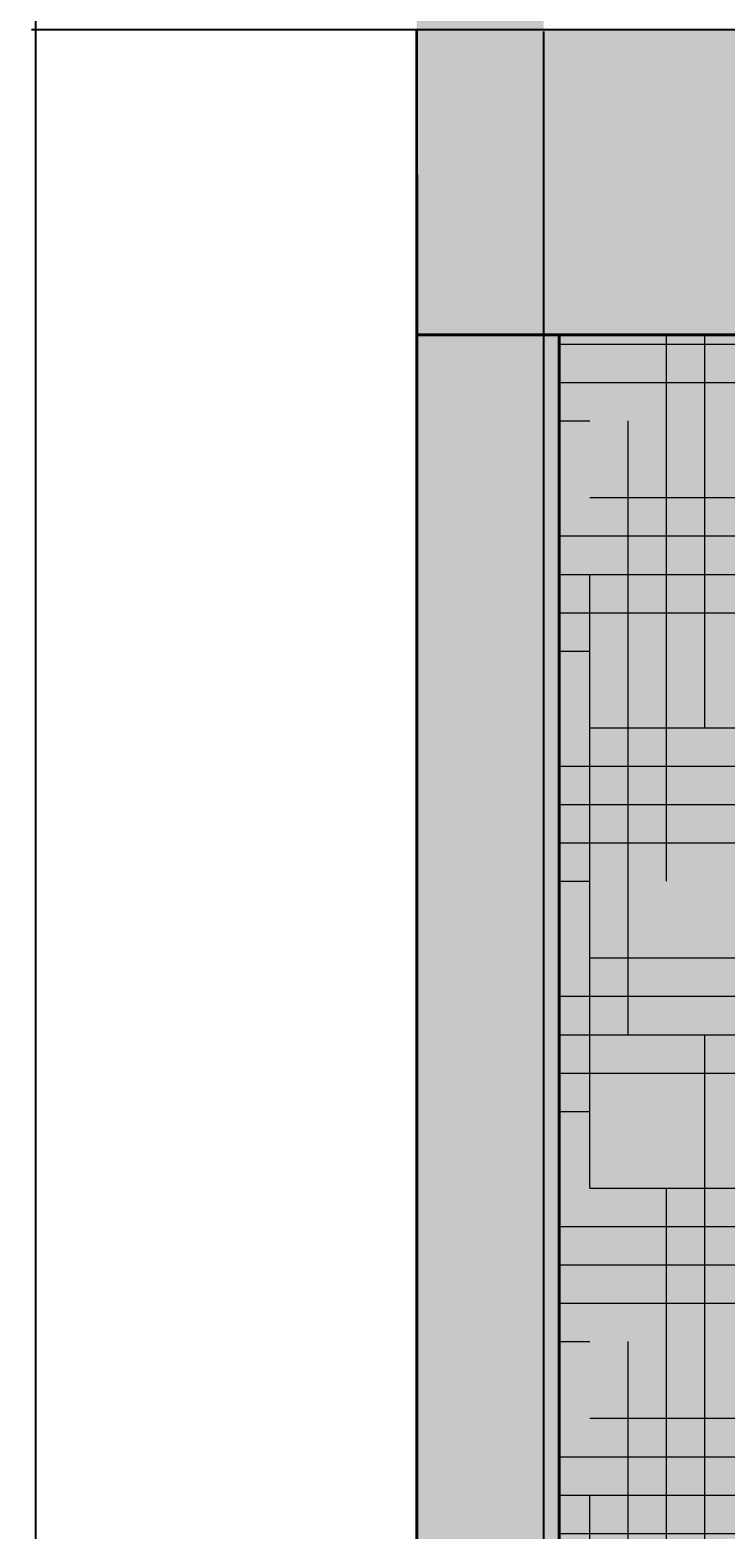
# Model space of a CAD drawing. Units: feet. Extents: x 2695 to 2912, y 795 to 1139.
# Tile 10 of 83: x 2695 to 2723, y 875 to 937. Entities that reach past the tile are written whole.
import ezdxf

# ---------------------------------------------------------------- set-up
doc = ezdxf.new("R2010")
doc.units = ezdxf.units.FT
for name, color, linetype, lineweight in [('A-ANNO-DIMS', 2, 'Continuous', 18), ('A-ELEV', 7, 'Continuous', 35), ('A-ELEV-PATT', 252, 'Continuous', 13)]:
    doc.layers.add(name, color=color, linetype=linetype, lineweight=lineweight)
doc.styles.get("Standard").update_dxf_attribs({"font": 'arial.ttf'})
doc.dimstyles.get("Standard").update_dxf_attribs({"dimtxt": 0.18, "dimasz": 0.18, "dimexe": 0.18, "dimexo": 0.0625, "dimgap": 0.09, "dimtad": 0, "dimtih": 1, "dimtoh": 1, "dimdec": 1, "dimzin": 0, "dimdsep": 46, "dimlunit": 3, "dimtxsty": 'Standard', "dimcen": 0.09, "dimadec": 0, "dimazin": 0, "dimtfac": 1, "dimtdec": 1, "dimtofl": 0, "dimtmove": 0, "dimatfit": 3, "dimfxl": 1, "dimtolj": 1, "dimtzin": 0, "dimarcsym": 0})

# ---------------------------------------------------------------- blocks, each defined once
blk = doc.blocks.new('*D12')
at = {"layer": 'A-ANNO-DIMS', "color": 0, "lineweight": -2, "transparency": 16777216}
for p, q in [((2710.574, 1122.931), (2694.681, 1122.931)), ((2694.861, 1122.751), (2694.861, 967.113)), ((2694.861, 811.111), (2694.861, 966.749)), ((2710.574, 810.931), (2694.681, 810.931))]:
    blk.add_line(p, q, dxfattribs=at)
at = {"layer": 'A-ANNO-DIMS', "color": 0, "transparency": 16777216}
for points in [[(2694.831, 1122.751), (2694.891, 1122.751), (2694.861, 1122.931)], [(2694.831, 811.111), (2694.891, 811.111), (2694.861, 810.931)]]:
    blk.add_solid(points, dxfattribs=at)
at = {"layer": 'Defpoints', "color": 0, "transparency": 16777216}
for p in [(2694.861, 1122.931), (2710.636, 1122.931), (2710.636, 810.931)]:
    blk.add_point(p, dxfattribs=at)
at = {"layer": 'A-ANNO-DIMS', "color": 0, "transparency": 16777216, "insert": (2694.861, 966.931), "char_height": 0.18, "attachment_point": 5}
blk.add_mtext('\\A1;312', dxfattribs=at)
blk = doc.blocks.new('*D23')
at = {"layer": 'A-ANNO-DIMS', "color": 0, "lineweight": -2, "transparency": 16777216}
for p, q in [((2715.885, 936.868), (2715.885, 794.976)), ((2730.708, 936.868), (2730.708, 794.976)), ((2716.065, 795.156), (2722.842, 795.156)), ((2730.528, 795.156), (2723.752, 795.156))]:
    blk.add_line(p, q, dxfattribs=at)
at = {"layer": 'A-ANNO-DIMS', "color": 0, "transparency": 16777216}
for points in [[(2716.065, 795.186), (2716.065, 795.126), (2715.885, 795.156)], [(2730.528, 795.186), (2730.528, 795.126), (2730.708, 795.156)]]:
    blk.add_solid(points, dxfattribs=at)
at = {"layer": 'Defpoints', "color": 0, "transparency": 16777216}
for p in [(2715.885, 936.931), (2730.708, 936.931), (2730.708, 795.156)]:
    blk.add_point(p, dxfattribs=at)
at = {"layer": 'A-ANNO-DIMS', "color": 0, "transparency": 16777216, "insert": (2723.297, 795.156), "char_height": 0.18, "attachment_point": 5}
blk.add_mtext('\\A1;14.823', dxfattribs=at)
blk = doc.blocks.new('*D27')
at = {"layer": 'A-ANNO-DIMS', "color": 0, "lineweight": -2, "transparency": 16777216}
for p, q in [((2730.646, 938.518), (2694.681, 938.518)), ((2694.861, 938.338), (2694.861, 937.906)), ((2694.861, 937.111), (2694.861, 937.542)), ((2730.646, 936.931), (2694.681, 936.931))]:
    blk.add_line(p, q, dxfattribs=at)
at = {"layer": 'A-ANNO-DIMS', "color": 0, "transparency": 16777216}
for points in [[(2694.831, 938.338), (2694.891, 938.338), (2694.861, 938.518)], [(2694.831, 937.111), (2694.891, 937.111), (2694.861, 936.931)]]:
    blk.add_solid(points, dxfattribs=at)
at = {"layer": 'Defpoints', "color": 0, "transparency": 16777216}
for p in [(2694.861, 938.518), (2730.708, 938.518), (2730.708, 936.931)]:
    blk.add_point(p, dxfattribs=at)
at = {"layer": 'A-ANNO-DIMS', "color": 0, "transparency": 16777216, "insert": (2694.861, 937.724), "char_height": 0.18, "attachment_point": 5}
blk.add_mtext('\\A1;1.59', dxfattribs=at)

msp = doc.modelspace()

# ---------------------------------------------------------------- hatches: boundary and pattern name
at = {"layer": 'A-ELEV-PATT'}
h = msp.add_hatch(color=256, dxfattribs=at)
h.set_gradient(color1=(255, 255, 255), tint=1)
h.paths.add_polyline_path([(2770.6361, 1122.9306), (2710.6361, 1122.9306), (2710.6361, 1118.4096), (2770.6361, 1118.4096)])
h.paths.add_polyline_path([(2890.6361, 1107.8588), (2770.6361, 1107.8588), (2770.6361, 1103.3378), (2890.6361, 1103.3378)])
h.paths.add_polyline_path([(2890.6361, 1062.9306), (2710.6361, 1062.9306), (2710.6361, 1056.9306), (2710.6361, 936.9306), (2710.6361, 924.3105), (2716.5358, 924.3105), (2890.6361, 924.3105), (2890.6361, 936.9306), (2715.8852, 936.9306), (2715.8852, 1050.3105), (2890.6361, 1050.3105)])
h.paths.add_polyline_path([(2716.5358, 924.3105), (2710.6361, 924.3105), (2710.6361, 810.9306), (2716.5358, 810.9306)])
h = msp.add_hatch(color=256, dxfattribs=at)
h.set_gradient(color1=(255, 255, 255))
h.paths.add_polyline_path([(2770.6361, 924.3105), (2716.5358, 924.3105), (2716.5358, 810.9306), (2770.6361, 810.9306)])
h.paths.add_polyline_path([(2758.1515, 902.577), (2758.1515, 874.8571), (2724.1893, 874.8571), (2724.1893, 902.577)], flags=16)
h.paths.add_polyline_path([(2756.1515, 900.577), (2756.1515, 876.8571), (2726.1893, 876.8571), (2726.1893, 900.577)], flags=0)
h.paths.add_polyline_path([(2740.7302, 900.577), (2741.6105, 900.577), (2741.6105, 876.8571), (2740.7302, 876.8571)], flags=0)
h = msp.add_hatch(dxfattribs=at)
h.set_pattern_fill('HOUND', color=256, style=0)
h.paths.add_polyline_path([(2770.6361, 924.3105), (2716.5358, 924.3105), (2716.5358, 810.9306), (2770.6361, 810.9306)])
h.paths.add_polyline_path([(2724.1893, 874.8571), (2724.1893, 902.577), (2758.1515, 902.577), (2758.1515, 874.8571)], flags=16)
h.paths.add_polyline_path([(2756.1515, 876.8571), (2726.1893, 876.8571), (2726.1893, 900.577), (2756.1515, 900.577)], flags=0)
h.paths.add_polyline_path([(2741.6105, 876.8571), (2740.7302, 876.8571), (2740.7302, 900.577), (2741.6105, 900.577)], flags=0)

# ---------------------------------------------------------------- linework, layer by layer
at = {"layer": 'A-ELEV'}
for p, q in [((2710.6361, 930.9306), (2710.6361, 936.9306)), ((2710.6361, 930.9306), (2710.6361, 810.9306)), ((2770.6361, 924.3105), (2716.5358, 924.3105)), ((2716.5358, 924.3105), (2716.5358, 810.9306))]:
    msp.add_line(p, q, dxfattribs=at)
msp.add_lwpolyline([(2890.6361, 936.9306), (2890.6361, 924.3105), (2710.6361, 924.3105), (2710.6361, 936.9306)], dxfattribs=at)
for points in [[(2710.6361, 924.3105), (2716.5358, 924.3105), (2716.5358, 810.9306), (2710.6361, 810.9306)], [(2716.5358, 924.3105), (2770.6361, 924.3105), (2770.6361, 810.9306), (2716.5358, 810.9306)]]:
    msp.add_lwpolyline(points, close=True, dxfattribs=at)

# ---------------------------------------------------------------- dimensions: what is measured, and where the dimension line sits
at = {"layer": 'A-ANNO-DIMS'}
for base, p1, p2, override, picture, middle in [((2694.8611, 1122.9306), (2710.6361, 810.9306), (2710.6361, 1122.9306), {"dimdec": 0, "dimlfac": 1, "dimrnd": 0, "dimzin": 0, "dimdsep": 46, "dimlunit": 2}, '*D12', (2694.8611, 966.9306)), ((2694.8611, 938.5179), (2730.7081, 936.9306), (2730.7081, 938.5179), {"dimdec": 2, "dimlfac": 1, "dimrnd": 0, "dimzin": 0, "dimdsep": 46, "dimlunit": 2}, '*D27', (2694.8611, 937.7242))]:
    dim = msp.add_linear_dim(base=base, p1=p1, p2=p2, angle=90, dimstyle='Standard', override=override, dxfattribs=at)
    dim.commit()
    dim.dimension.update_dxf_attribs({"geometry": picture, "text_midpoint": middle})
dim = msp.add_linear_dim(base=(2730.7081, 795.1556), p1=(2715.8852, 936.9306), p2=(2730.7081, 936.9306), dimstyle='Standard', override={"dimdec": 3, "dimlfac": 1, "dimrnd": 0, "dimzin": 0, "dimdsep": 46, "dimlunit": 2}, dxfattribs=at)
dim.commit()
dim.dimension.update_dxf_attribs({"geometry": '*D23', "text_midpoint": (2723.2967, 795.1556)})

doc.saveas('drawing.dxf')
